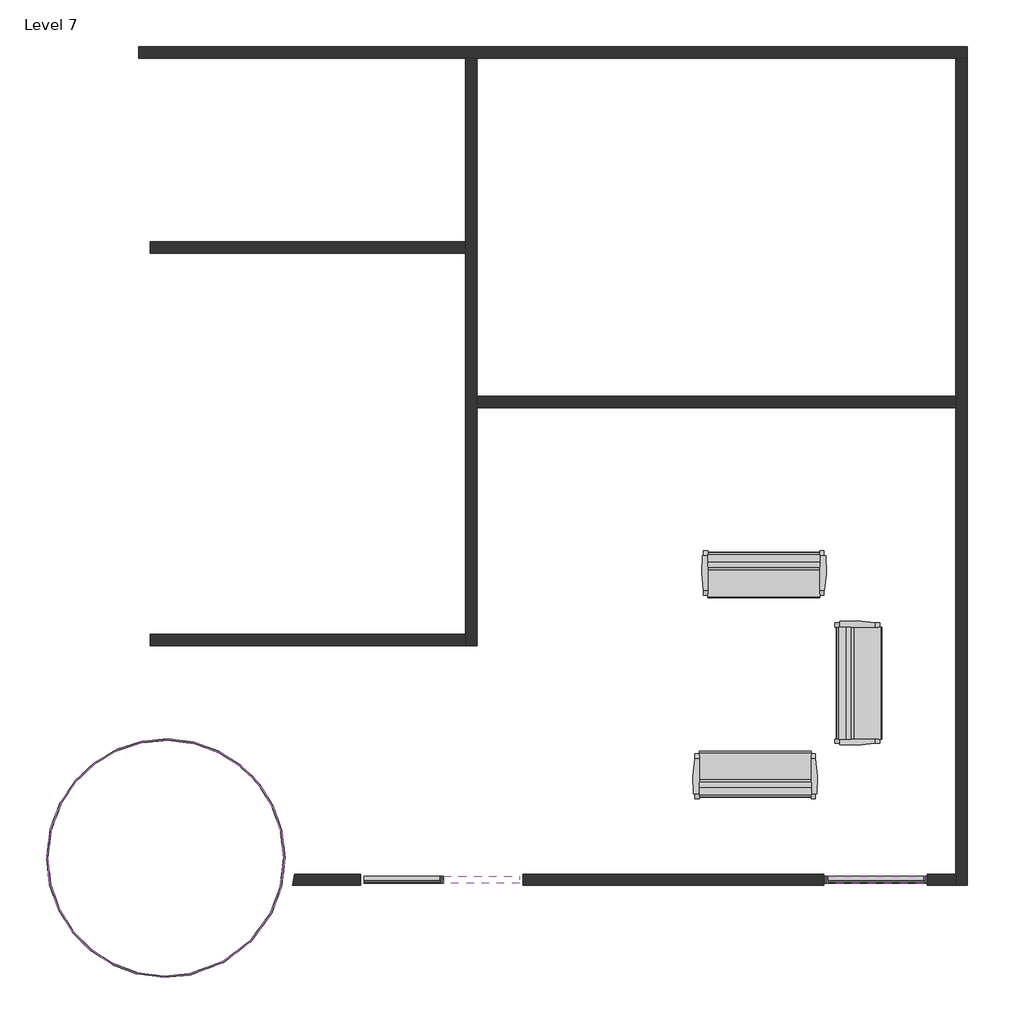
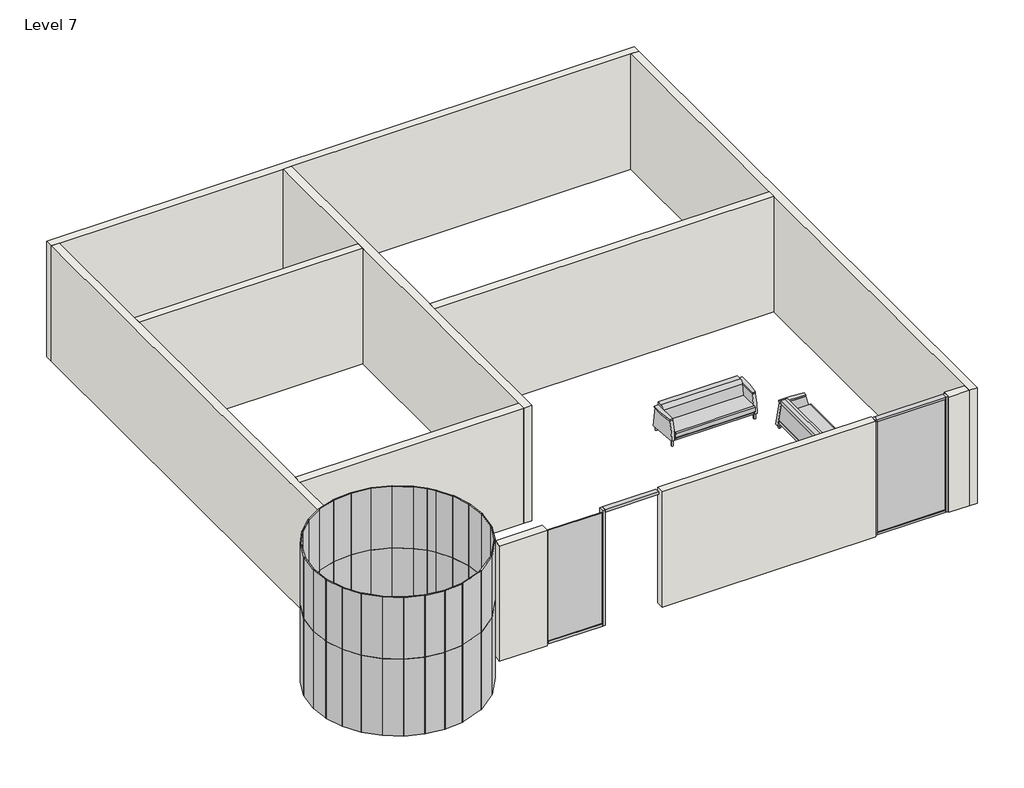
# One storey, incomplete: 58 plates, 10 walls, 7 members, 3 furniture elements.
"""IFC4 building model written with IfcOpenShell, lengths in millimetres."""

from ifc_helpers import new_model, si_unit, point, frame, frame_2d, origin, place, context, project, spatial, polyline, circle_curve, trimmed, segment, composite_curve, outline, extrude, faceted_brep, transform, mapped, element, save
from ifc_brep_helpers import plane_surface, revolved_surface, advanced_brep
from components import furniture_aff9b2fb, member_eaba9652, member_3f395ae9, member_0c868e12, member_7bc42366, system_panel_glazed_f1c144f9, system_panel_glazed_8ed2b2ee, system_panel_glazed_c7815b78, system_panel_glazed_220ba5f3, system_panel_glazed_11fb153e, system_panel_glazed_2f540b85, system_panel_glazed_4848e608, system_panel_glazed_8b35a0ff, system_panel_glazed_87282c25, system_panel_glazed_6d1bb68c, system_panel_glazed_cb3ffd69, system_panel_glazed_404d015f, system_panel_glazed_7b556abe, system_panel_glazed_370bf902

model = new_model("IFC4")

# Units and contexts
model_context = context("Model", 3, world=origin())
ifc_project = project(units=[si_unit("LENGTHUNIT", "METRE", prefix="MILLI")], contexts=[model_context])

# Site, building, storey
site = spatial("IfcSite", under=ifc_project)
building = spatial("IfcBuilding", under=site)
storey = spatial("IfcBuildingStorey", under=building, Name="Level 7", Elevation=18288.0)

# Furniture
placement = place(None, origin())
furniture_shape = furniture_aff9b2fb(model_context)
element("IfcFurniture", 1, ObjectType="Sofa-Pensi : 84\"", at=placement, inside=storey, context=model_context, shape_type="MappedRepresentation", body=[
    mapped(furniture_shape, transform((-2244.8524991, 3650.1964615, 18288.0), x_axis=(1.0, 0.0, 0.0), y_axis=(0.0, 1.0, 0.0), z_axis=(0.0, 0.0, 1.0))),
])
element("IfcFurniture", 2, ObjectType="Sofa-Pensi : 84\"", at=placement, inside=storey, context=model_context, shape_type="MappedRepresentation", body=[
    mapped(furniture_shape, transform((-12.736413, 1720.492712, 18288.0), x_axis=(0.0, 1.0, 0.0), y_axis=(-1.0, 0.0, 0.0), z_axis=(0.0, 0.0, 1.0))),
])
element("IfcFurniture", 3, ObjectType="Sofa-Pensi : 84\"", at=placement, inside=storey, context=model_context, shape_type="MappedRepresentation", body=[
    mapped(furniture_shape, transform((-1840.0399991, 648.4161336, 18288.0), x_axis=(-1.0, 0.0, 0.0), y_axis=(0.0, -1.0, 0.0), z_axis=(0.0, 0.0, 1.0))),
])

# Members
member_shape = member_eaba9652(model_context)
element("IfcMember", 4, ObjectType="Rectangular Mullion : 2.5\" x 5\" rectangular", at=placement, inside=storey, context=model_context, shape_type="MappedRepresentation", body=[
    mapped(member_shape, transform((-7672.5789001, -1482.8937024, 18288.0), x_axis=(-1.0, 0.0, 0.0), y_axis=(0.0, 1.0, 0.0), z_axis=(0.0, 0.0, -1.0))),
])
member_2_shape = member_3f395ae9(model_context)
element("IfcMember", 5, ObjectType="Rectangular Mullion : 2.5\" x 5\" rectangular", at=placement, inside=storey, context=model_context, shape_type="MappedRepresentation", body=[
    mapped(member_2_shape, transform((-899.4462491, -1482.8937024, 18288.0), x_axis=(-1.0, 0.0, 0.0), y_axis=(0.0, 1.0, 0.0), z_axis=(0.0, 0.0, -1.0))),
])
element("IfcMember", 6, ObjectType="Rectangular Mullion : 2.5\" x 5\" rectangular", at=placement, inside=storey, context=model_context, shape_type="MappedRepresentation", body=[
    mapped(member_2_shape, transform((929.3537509, -1482.8937024, 21336.0), x_axis=(1.0, 0.0, 0.0), y_axis=(0.0, 1.0, 0.0), z_axis=(0.0, 0.0, 1.0))),
])
member_3_shape = member_0c868e12(model_context)
element("IfcMember", 7, ObjectType="Rectangular Mullion : 2.5\" x 5\" rectangular", at=placement, inside=storey, context=model_context, shape_type="MappedRepresentation", body=[
    mapped(member_3_shape, transform((-7640.8289001, -1482.8937024, 21336.0), x_axis=(0.0, 0.0, 1.0), y_axis=(0.0, 1.0, 0.0), z_axis=(-1.0, 0.0, 0.0))),
])
element("IfcMember", 8, ObjectType="Rectangular Mullion : 2.5\" x 5\" rectangular", at=placement, inside=storey, context=model_context, shape_type="MappedRepresentation", body=[
    mapped(member_3_shape, transform((-7704.3289001, -1482.8937024, 18288.0), x_axis=(0.0, 0.0, -1.0), y_axis=(0.0, 1.0, 0.0), z_axis=(1.0, 0.0, 0.0))),
])
member_4_shape = member_7bc42366(model_context)
element("IfcMember", 9, ObjectType="Rectangular Mullion : 2.5\" x 5\" rectangular", at=placement, inside=storey, context=model_context, shape_type="MappedRepresentation", body=[
    mapped(member_4_shape, transform((-835.9462491, -1482.8937024, 21336.0), x_axis=(0.0, 0.0, 1.0), y_axis=(0.0, 1.0, 0.0), z_axis=(-1.0, 0.0, 0.0))),
])
element("IfcMember", 10, ObjectType="Rectangular Mullion : 2.5\" x 5\" rectangular", at=placement, inside=storey, context=model_context, shape_type="MappedRepresentation", body=[
    mapped(member_4_shape, transform((865.8537509, -1482.8937024, 18288.0), x_axis=(0.0, 0.0, -1.0), y_axis=(0.0, 1.0, 0.0), z_axis=(1.0, 0.0, 0.0))),
])

# Plates
system_panel_glazed_shape = system_panel_glazed_f1c144f9(model_context)
element("IfcPlate", 11, ObjectType="System Panel : Glazed", at=placement, inside=storey, context=model_context, shape_type="MappedRepresentation", body=[
    mapped(system_panel_glazed_shape, transform((-14541.9245022, -346.5978939, 18288.0), x_axis=(-0.3551689475306269, -0.9348021281051873, 0.0), y_axis=(0.9348021281051873, -0.3551689475306269, 0.0), z_axis=(0.0, 0.0, 1.0))),
])
element("IfcPlate", 12, ObjectType="System Panel : Glazed", at=placement, inside=storey, context=model_context, shape_type="MappedRepresentation", body=[
    mapped(system_panel_glazed_shape, transform((-10582.1178502, -1851.0877948, 18288.0), x_axis=(0.35516894753064066, 0.934802128105182, 0.0), y_axis=(-0.934802128105182, 0.35516894753064066, 0.0), z_axis=(0.0, 0.0, 1.0))),
])
element("IfcPlate", 13, ObjectType="System Panel : Glazed", at=placement, inside=storey, context=model_context, shape_type="MappedRepresentation", body=[
    mapped(system_panel_glazed_shape, transform((-10459.5232171, -1354.5613954, 18288.0), x_axis=(0.12073632210407237, 0.9926846128175765, 0.0), y_axis=(-0.9926846128175765, 0.12073632210407237, 0.0), z_axis=(0.0, 0.0, 1.0))),
])
element("IfcPlate", 14, ObjectType="System Panel : Glazed", at=placement, inside=storey, context=model_context, shape_type="MappedRepresentation", body=[
    mapped(system_panel_glazed_shape, transform((-14664.5191354, -843.1242933, 18288.0), x_axis=(-0.12073632210406239, -0.9926846128175777, 0.0), y_axis=(0.9926846128175777, -0.12073632210406239, 0.0), z_axis=(0.0, 0.0, 1.0))),
])
system_panel_glazed_2_shape = system_panel_glazed_8ed2b2ee(model_context)
element("IfcPlate", 15, ObjectType="System Panel : Glazed", at=placement, inside=storey, context=model_context, shape_type="MappedRepresentation", body=[
    mapped(system_panel_glazed_2_shape, transform((-11841.3777431, -3082.3793017, 18288.0), x_axis=(0.9398911711666007, 0.3414741371803665, 0.0), y_axis=(-0.3414741371803665, 0.9398911711666007, 0.0), z_axis=(0.0, 0.0, 1.0))),
])
element("IfcPlate", 16, ObjectType="System Panel : Glazed", at=placement, inside=storey, context=model_context, shape_type="MappedRepresentation", body=[
    mapped(system_panel_glazed_2_shape, transform((-10858.9635423, -2345.1728692, 18288.0), x_axis=(0.5905687200141164, 0.8069873524045393, 0.0), y_axis=(-0.8069873524045393, 0.5905687200141164, 0.0), z_axis=(0.0, 0.0, 1.0))),
])
element("IfcPlate", 17, ObjectType="System Panel : Glazed", at=placement, inside=storey, context=model_context, shape_type="MappedRepresentation", body=[
    mapped(system_panel_glazed_2_shape, transform((-11295.3522982, -2786.8279712, 18288.0), x_axis=(0.7998453025525061, 0.6002062078858317, 0.0), y_axis=(-0.6002062078858317, 0.7998453025525061, 0.0), z_axis=(0.0, 0.0, 1.0))),
])
system_panel_glazed_3_shape = system_panel_glazed_c7815b78(model_context)
element("IfcPlate", 18, ObjectType="System Panel : Glazed", at=placement, inside=storey, context=model_context, shape_type="MappedRepresentation", body=[
    mapped(system_panel_glazed_3_shape, transform((-10454.4737362, -864.5204039, 18288.0), x_axis=(-0.11050163420416614, 0.993875942378227, 0.0), y_axis=(-0.993875942378227, -0.11050163420416614, 0.0), z_axis=(0.0, 0.0, 1.0))),
])
element("IfcPlate", 19, ObjectType="System Panel : Glazed", at=placement, inside=storey, context=model_context, shape_type="MappedRepresentation", body=[
    mapped(system_panel_glazed_3_shape, transform((-14669.5686163, -1333.1652848, 18288.0), x_axis=(0.11050163420415136, -0.9938759423782286, 0.0), y_axis=(0.9938759423782286, 0.11050163420415136, 0.0), z_axis=(0.0, 0.0, 1.0))),
])
element("IfcPlate", 20, ObjectType="System Panel : Glazed", at=placement, inside=storey, context=model_context, shape_type="MappedRepresentation", body=[
    mapped(system_panel_glazed_3_shape, transform((-11410.1424167, 681.5611944, 18288.0), x_axis=(-0.8396018558176894, 0.5432022861766066, 0.0), y_axis=(-0.5432022861766066, -0.8396018558176894, 0.0), z_axis=(0.0, 0.0, 1.0))),
])
element("IfcPlate", 21, ObjectType="System Panel : Glazed", at=placement, inside=storey, context=model_context, shape_type="MappedRepresentation", body=[
    mapped(system_panel_glazed_3_shape, transform((-13212.0893695, 919.590846, 18288.0), x_axis=(-0.9518517343814786, -0.3065587639506839, 0.0), y_axis=(0.3065587639506839, -0.9518517343814786, 0.0), z_axis=(0.0, 0.0, 1.0))),
])
element("IfcPlate", 22, ObjectType="System Panel : Glazed", at=placement, inside=storey, context=model_context, shape_type="MappedRepresentation", body=[
    mapped(system_panel_glazed_3_shape, transform((-12839.7224363, -3201.1142893, 18288.0), x_axis=(0.9913878918151698, -0.1309581916577702, 0.0), y_axis=(0.1309581916577702, 0.9913878918151698, 0.0), z_axis=(0.0, 0.0, 1.0))),
])
element("IfcPlate", 23, ObjectType="System Panel : Glazed", at=placement, inside=storey, context=model_context, shape_type="MappedRepresentation", body=[
    mapped(system_panel_glazed_3_shape, transform((-14365.783041, -2213.7896382, 18288.0), x_axis=(0.5257859322352114, -0.8506169252157811, 0.0), y_axis=(0.8506169252157811, 0.5257859322352114, 0.0), z_axis=(0.0, 0.0, 1.0))),
])
element("IfcPlate", 24, ObjectType="System Panel : Glazed", at=placement, inside=storey, context=model_context, shape_type="MappedRepresentation", body=[
    mapped(system_panel_glazed_3_shape, transform((-13713.8999358, -2879.2468831, 18288.0), x_axis=(0.8396018558176805, -0.5432022861766201, 0.0), y_axis=(0.5432022861766201, 0.8396018558176805, 0.0), z_axis=(0.0, 0.0, 1.0))),
])
element("IfcPlate", 25, ObjectType="System Panel : Glazed", at=placement, inside=storey, context=model_context, shape_type="MappedRepresentation", body=[
    mapped(system_panel_glazed_3_shape, transform((-14014.4059364, 446.2272921, 18288.0), x_axis=(-0.7286232370002992, -0.6849147235263715, 0.0), y_axis=(0.6849147235263715, -0.7286232370002992, 0.0), z_axis=(0.0, 0.0, 1.0))),
])
element("IfcPlate", 26, ObjectType="System Panel : Glazed", at=placement, inside=storey, context=model_context, shape_type="MappedRepresentation", body=[
    mapped(system_panel_glazed_3_shape, transform((-12284.3199161, 1003.4286006, 18288.0), x_axis=(-0.9913878918151723, 0.13095819165775144, 0.0), y_axis=(-0.13095819165775144, -0.9913878918151723, 0.0), z_axis=(0.0, 0.0, 1.0))),
])
element("IfcPlate", 27, ObjectType="System Panel : Glazed", at=placement, inside=storey, context=model_context, shape_type="MappedRepresentation", body=[
    mapped(system_panel_glazed_3_shape, transform((-12752.8652893, 1013.0855973, 18288.0), x_axis=(-0.9959419324521102, -0.08999815100076568, 0.0), y_axis=(0.08999815100076568, -0.9959419324521102, 0.0), z_axis=(0.0, 0.0, 1.0))),
])
element("IfcPlate", 28, ObjectType="System Panel : Glazed", at=placement, inside=storey, context=model_context, shape_type="MappedRepresentation", body=[
    mapped(system_panel_glazed_3_shape, transform((-11829.3381514, 891.0915272, 18288.0), x_axis=(-0.9384120429483949, 0.3455182160891376, 0.0), y_axis=(-0.3455182160891376, -0.9384120429483949, 0.0), z_axis=(0.0, 0.0, 1.0))),
])
element("IfcPlate", 29, ObjectType="System Panel : Glazed", at=placement, inside=storey, context=model_context, shape_type="MappedRepresentation", body=[
    mapped(system_panel_glazed_3_shape, transform((-10557.4115054, -407.3204039, 18288.0), x_axis=(-0.3261077326604367, 0.9453326116764772, 0.0), y_axis=(-0.9453326116764772, -0.3261077326604367, 0.0), z_axis=(0.0, 0.0, 1.0))),
])
element("IfcPlate", 30, ObjectType="System Panel : Glazed", at=placement, inside=storey, context=model_context, shape_type="MappedRepresentation", body=[
    mapped(system_panel_glazed_3_shape, transform((-12371.1770631, -3210.771286, 18288.0), x_axis=(0.9959419324521115, 0.08999815100075001, 0.0), y_axis=(-0.08999815100075001, 0.9959419324521115, 0.0), z_axis=(0.0, 0.0, 1.0))),
])
element("IfcPlate", 31, ObjectType="System Panel : Glazed", at=placement, inside=storey, context=model_context, shape_type="MappedRepresentation", body=[
    mapped(system_panel_glazed_3_shape, transform((-13294.7042011, -3088.7772159, 18288.0), x_axis=(0.9384120429483891, -0.34551821608915334, 0.0), y_axis=(0.34551821608915334, 0.9384120429483891, 0.0), z_axis=(0.0, 0.0, 1.0))),
])
element("IfcPlate", 32, ObjectType="System Panel : Glazed", at=placement, inside=storey, context=model_context, shape_type="MappedRepresentation", body=[
    mapped(system_panel_glazed_3_shape, transform((-14076.8350959, -2582.7572647, 18288.0), x_axis=(0.6997834615185511, -0.7143550286692988, 0.0), y_axis=(0.7143550286692988, 0.6997834615185511, 0.0), z_axis=(0.0, 0.0, 1.0))),
])
element("IfcPlate", 33, ObjectType="System Panel : Glazed", at=placement, inside=storey, context=model_context, shape_type="MappedRepresentation", body=[
    mapped(system_panel_glazed_3_shape, transform((-14566.6308471, -1790.3652848, 18288.0), x_axis=(0.32610773266042153, -0.9453326116764824, 0.0), y_axis=(0.9453326116764824, 0.32610773266042153, 0.0), z_axis=(0.0, 0.0, 1.0))),
])
element("IfcPlate", 34, ObjectType="System Panel : Glazed", at=placement, inside=storey, context=model_context, shape_type="MappedRepresentation", body=[
    mapped(system_panel_glazed_3_shape, transform((-14318.3113206, 89.4787227, 18288.0), x_axis=(-0.5603879632167612, -0.8282302401396425, 0.0), y_axis=(0.8282302401396425, -0.5603879632167612, 0.0), z_axis=(0.0, 0.0, 1.0))),
])
element("IfcPlate", 35, ObjectType="System Panel : Glazed", at=placement, inside=storey, context=model_context, shape_type="MappedRepresentation", body=[
    mapped(system_panel_glazed_3_shape, transform((-13639.5625299, 727.5108588, 18288.0), x_axis=(-0.8612707706620224, -0.5081462974412448, 0.0), y_axis=(0.5081462974412448, -0.8612707706620224, 0.0), z_axis=(0.0, 0.0, 1.0))),
])
system_panel_glazed_4_shape = system_panel_glazed_220ba5f3(model_context)
element("IfcPlate", 36, ObjectType="System Panel : Glazed", at=placement, inside=storey, context=model_context, shape_type="MappedRepresentation", body=[
    mapped(system_panel_glazed_4_shape, transform((-10742.3305673, -4.7597883, 18288.0), x_axis=(-0.5152811917631037, 0.8570211744263939, 0.0), y_axis=(-0.8570211744263939, -0.5152811917631037, 0.0), z_axis=(0.0, 0.0, 1.0))),
])
system_panel_glazed_5_shape = system_panel_glazed_11fb153e(model_context)
element("IfcPlate", 37, ObjectType="System Panel : Glazed", at=placement, inside=storey, context=model_context, shape_type="MappedRepresentation", body=[
    mapped(system_panel_glazed_5_shape, transform((-11098.0043985, 445.2241463, 18288.0), x_axis=(-0.7256671855033587, 0.6880458821064435, 0.0), y_axis=(-0.6880458821064435, -0.7256671855033587, 0.0), z_axis=(0.0, 0.0, 1.0))),
])
system_panel_glazed_6_shape = system_panel_glazed_2f540b85(model_context)
element("IfcPlate", 38, ObjectType="System Panel : Glazed", at=placement, inside=storey, context=model_context, shape_type="MappedRepresentation", body=[
    mapped(system_panel_glazed_6_shape, transform((-10917.0903061, 255.9395759, 18288.0), x_axis=(-0.6357445726375757, 0.7718995001694627, 0.0), y_axis=(-0.7718995001694627, -0.6357445726375757, 0.0), z_axis=(0.0, 0.0, 1.0))),
])
system_panel_glazed_7_shape = system_panel_glazed_4848e608(model_context)
element("IfcPlate", 39, ObjectType="System Panel : Glazed", at=placement, inside=storey, context=model_context, shape_type="MappedRepresentation", body=[
    mapped(system_panel_glazed_7_shape, transform((-14669.5686163, -1333.1652848, 20320.0), x_axis=(0.11050163420415136, -0.9938759423782286, 0.0), y_axis=(0.9938759423782286, 0.11050163420415136, 0.0), z_axis=(0.0, 0.0, 1.0))),
])
element("IfcPlate", 40, ObjectType="System Panel : Glazed", at=placement, inside=storey, context=model_context, shape_type="MappedRepresentation", body=[
    mapped(system_panel_glazed_7_shape, transform((-14365.783041, -2213.7896382, 20320.0), x_axis=(0.5257859322352114, -0.8506169252157811, 0.0), y_axis=(0.8506169252157811, 0.5257859322352114, 0.0), z_axis=(0.0, 0.0, 1.0))),
])
element("IfcPlate", 41, ObjectType="System Panel : Glazed", at=placement, inside=storey, context=model_context, shape_type="MappedRepresentation", body=[
    mapped(system_panel_glazed_7_shape, transform((-13713.8999358, -2879.2468831, 20320.0), x_axis=(0.8396018558176805, -0.5432022861766201, 0.0), y_axis=(0.5432022861766201, 0.8396018558176805, 0.0), z_axis=(0.0, 0.0, 1.0))),
])
element("IfcPlate", 42, ObjectType="System Panel : Glazed", at=placement, inside=storey, context=model_context, shape_type="MappedRepresentation", body=[
    mapped(system_panel_glazed_7_shape, transform((-12839.7224363, -3201.1142893, 20320.0), x_axis=(0.9913878918151698, -0.13095819165777017, 0.0), y_axis=(0.13095819165777017, 0.9913878918151698, 0.0), z_axis=(0.0, 0.0, 1.0))),
])
element("IfcPlate", 43, ObjectType="System Panel : Glazed", at=placement, inside=storey, context=model_context, shape_type="MappedRepresentation", body=[
    mapped(system_panel_glazed_7_shape, transform((-12371.1770631, -3210.771286, 20320.0), x_axis=(0.9959419324521115, 0.08999815100075001, 0.0), y_axis=(-0.08999815100075001, 0.9959419324521115, 0.0), z_axis=(0.0, 0.0, 1.0))),
])
element("IfcPlate", 44, ObjectType="System Panel : Glazed", at=placement, inside=storey, context=model_context, shape_type="MappedRepresentation", body=[
    mapped(system_panel_glazed_7_shape, transform((-13294.7042011, -3088.7772159, 20320.0), x_axis=(0.9384120429483891, -0.34551821608915334, 0.0), y_axis=(0.34551821608915334, 0.9384120429483891, 0.0), z_axis=(0.0, 0.0, 1.0))),
])
element("IfcPlate", 45, ObjectType="System Panel : Glazed", at=placement, inside=storey, context=model_context, shape_type="MappedRepresentation", body=[
    mapped(system_panel_glazed_7_shape, transform((-14076.8350959, -2582.7572647, 20320.0), x_axis=(0.6997834615185511, -0.7143550286692988, 0.0), y_axis=(0.7143550286692988, 0.6997834615185511, 0.0), z_axis=(0.0, 0.0, 1.0))),
])
element("IfcPlate", 46, ObjectType="System Panel : Glazed", at=placement, inside=storey, context=model_context, shape_type="MappedRepresentation", body=[
    mapped(system_panel_glazed_7_shape, transform((-14566.6308471, -1790.3652848, 20320.0), x_axis=(0.32610773266042153, -0.9453326116764824, 0.0), y_axis=(0.9453326116764824, 0.32610773266042153, 0.0), z_axis=(0.0, 0.0, 1.0))),
])
element("IfcPlate", 47, ObjectType="System Panel : Glazed", at=placement, inside=storey, context=model_context, shape_type="MappedRepresentation", body=[
    mapped(system_panel_glazed_7_shape, transform((-10454.4737362, -864.5204039, 20320.0), x_axis=(-0.11050163420416614, 0.993875942378227, 0.0), y_axis=(-0.993875942378227, -0.11050163420416614, 0.0), z_axis=(0.0, 0.0, 1.0))),
])
element("IfcPlate", 48, ObjectType="System Panel : Glazed", at=placement, inside=storey, context=model_context, shape_type="MappedRepresentation", body=[
    mapped(system_panel_glazed_7_shape, transform((-10557.4115054, -407.3204039, 20320.0), x_axis=(-0.3261077326604368, 0.9453326116764772, 0.0), y_axis=(-0.9453326116764772, -0.3261077326604368, 0.0), z_axis=(0.0, 0.0, 1.0))),
])
element("IfcPlate", 49, ObjectType="System Panel : Glazed", at=placement, inside=storey, context=model_context, shape_type="MappedRepresentation", body=[
    mapped(system_panel_glazed_7_shape, transform((-11410.1424167, 681.5611944, 20320.0), x_axis=(-0.8396018558176894, 0.5432022861766066, 0.0), y_axis=(-0.5432022861766066, -0.8396018558176894, 0.0), z_axis=(0.0, 0.0, 1.0))),
])
element("IfcPlate", 50, ObjectType="System Panel : Glazed", at=placement, inside=storey, context=model_context, shape_type="MappedRepresentation", body=[
    mapped(system_panel_glazed_7_shape, transform((-11829.3381514, 891.0915272, 20320.0), x_axis=(-0.9384120429483949, 0.3455182160891376, 0.0), y_axis=(-0.3455182160891376, -0.9384120429483949, 0.0), z_axis=(0.0, 0.0, 1.0))),
])
element("IfcPlate", 51, ObjectType="System Panel : Glazed", at=placement, inside=storey, context=model_context, shape_type="MappedRepresentation", body=[
    mapped(system_panel_glazed_7_shape, transform((-12284.3199161, 1003.4286006, 20320.0), x_axis=(-0.9913878918151723, 0.1309581916577514, 0.0), y_axis=(-0.1309581916577514, -0.9913878918151723, 0.0), z_axis=(0.0, 0.0, 1.0))),
])
element("IfcPlate", 52, ObjectType="System Panel : Glazed", at=placement, inside=storey, context=model_context, shape_type="MappedRepresentation", body=[
    mapped(system_panel_glazed_7_shape, transform((-12752.8652893, 1013.0855973, 20320.0), x_axis=(-0.9959419324521102, -0.08999815100076568, 0.0), y_axis=(0.08999815100076568, -0.9959419324521102, 0.0), z_axis=(0.0, 0.0, 1.0))),
])
element("IfcPlate", 53, ObjectType="System Panel : Glazed", at=placement, inside=storey, context=model_context, shape_type="MappedRepresentation", body=[
    mapped(system_panel_glazed_7_shape, transform((-13212.0893695, 919.590846, 20320.0), x_axis=(-0.9518517343814786, -0.3065587639506839, 0.0), y_axis=(0.3065587639506839, -0.9518517343814786, 0.0), z_axis=(0.0, 0.0, 1.0))),
])
element("IfcPlate", 54, ObjectType="System Panel : Glazed", at=placement, inside=storey, context=model_context, shape_type="MappedRepresentation", body=[
    mapped(system_panel_glazed_7_shape, transform((-13639.5625299, 727.5108588, 20320.0), x_axis=(-0.8612707706620223, -0.508146297441245, 0.0), y_axis=(0.508146297441245, -0.8612707706620223, 0.0), z_axis=(0.0, 0.0, 1.0))),
])
element("IfcPlate", 55, ObjectType="System Panel : Glazed", at=placement, inside=storey, context=model_context, shape_type="MappedRepresentation", body=[
    mapped(system_panel_glazed_7_shape, transform((-14014.4059364, 446.2272921, 20320.0), x_axis=(-0.7286232370002992, -0.6849147235263715, 0.0), y_axis=(0.6849147235263715, -0.7286232370002992, 0.0), z_axis=(0.0, 0.0, 1.0))),
])
element("IfcPlate", 56, ObjectType="System Panel : Glazed", at=placement, inside=storey, context=model_context, shape_type="MappedRepresentation", body=[
    mapped(system_panel_glazed_7_shape, transform((-14318.3113206, 89.4787227, 20320.0), x_axis=(-0.5603879632167612, -0.8282302401396425, 0.0), y_axis=(0.8282302401396425, -0.5603879632167612, 0.0), z_axis=(0.0, 0.0, 1.0))),
])
system_panel_glazed_8_shape = system_panel_glazed_8b35a0ff(model_context)
element("IfcPlate", 57, ObjectType="System Panel : Glazed", at=placement, inside=storey, context=model_context, shape_type="MappedRepresentation", body=[
    mapped(system_panel_glazed_8_shape, transform((-10742.3305673, -4.7597883, 20320.0), x_axis=(-0.5152811917631037, 0.8570211744263939, 0.0), y_axis=(-0.8570211744263939, -0.5152811917631037, 0.0), z_axis=(0.0, 0.0, 1.0))),
])
system_panel_glazed_9_shape = system_panel_glazed_87282c25(model_context)
element("IfcPlate", 58, ObjectType="System Panel : Glazed", at=placement, inside=storey, context=model_context, shape_type="MappedRepresentation", body=[
    mapped(system_panel_glazed_9_shape, transform((-10917.0903061, 255.9395759, 20320.0), x_axis=(-0.6357445726375757, 0.7718995001694627, 0.0), y_axis=(-0.7718995001694627, -0.6357445726375757, 0.0), z_axis=(0.0, 0.0, 1.0))),
])
system_panel_glazed_10_shape = system_panel_glazed_6d1bb68c(model_context)
element("IfcPlate", 59, ObjectType="System Panel : Glazed", at=placement, inside=storey, context=model_context, shape_type="MappedRepresentation", body=[
    mapped(system_panel_glazed_10_shape, transform((-11098.0043985, 445.2241463, 20320.0), x_axis=(-0.7256671855033587, 0.6880458821064435, 0.0), y_axis=(-0.6880458821064435, -0.7256671855033587, 0.0), z_axis=(0.0, 0.0, 1.0))),
])
system_panel_glazed_11_shape = system_panel_glazed_cb3ffd69(model_context)
element("IfcPlate", 60, ObjectType="System Panel : Glazed", at=placement, inside=storey, context=model_context, shape_type="MappedRepresentation", body=[
    mapped(system_panel_glazed_11_shape, transform((-10582.1178502, -1851.0877948, 20320.0), x_axis=(0.35516894753064066, 0.934802128105182, 0.0), y_axis=(-0.934802128105182, 0.35516894753064066, 0.0), z_axis=(0.0, 0.0, 1.0))),
])
element("IfcPlate", 61, ObjectType="System Panel : Glazed", at=placement, inside=storey, context=model_context, shape_type="MappedRepresentation", body=[
    mapped(system_panel_glazed_11_shape, transform((-10459.5232171, -1354.5613954, 20320.0), x_axis=(0.1207363221040724, 0.9926846128175765, 0.0), y_axis=(-0.9926846128175765, 0.1207363221040724, 0.0), z_axis=(0.0, 0.0, 1.0))),
])
element("IfcPlate", 62, ObjectType="System Panel : Glazed", at=placement, inside=storey, context=model_context, shape_type="MappedRepresentation", body=[
    mapped(system_panel_glazed_11_shape, transform((-14541.9245022, -346.5978939, 20320.0), x_axis=(-0.3551689475306269, -0.9348021281051873, 0.0), y_axis=(0.9348021281051873, -0.3551689475306269, 0.0), z_axis=(0.0, 0.0, 1.0))),
])
element("IfcPlate", 63, ObjectType="System Panel : Glazed", at=placement, inside=storey, context=model_context, shape_type="MappedRepresentation", body=[
    mapped(system_panel_glazed_11_shape, transform((-14664.5191354, -843.1242933, 20320.0), x_axis=(-0.1207363221040624, -0.9926846128175777, 0.0), y_axis=(0.9926846128175777, -0.1207363221040624, 0.0), z_axis=(0.0, 0.0, 1.0))),
])
system_panel_glazed_12_shape = system_panel_glazed_404d015f(model_context)
element("IfcPlate", 64, ObjectType="System Panel : Glazed", at=placement, inside=storey, context=model_context, shape_type="MappedRepresentation", body=[
    mapped(system_panel_glazed_12_shape, transform((-11841.3777431, -3082.3793017, 20320.0), x_axis=(0.9398911711666007, 0.3414741371803665, 0.0), y_axis=(-0.3414741371803665, 0.9398911711666007, 0.0), z_axis=(0.0, 0.0, 1.0))),
])
element("IfcPlate", 65, ObjectType="System Panel : Glazed", at=placement, inside=storey, context=model_context, shape_type="MappedRepresentation", body=[
    mapped(system_panel_glazed_12_shape, transform((-10858.9635423, -2345.1728692, 20320.0), x_axis=(0.5905687200141164, 0.8069873524045393, 0.0), y_axis=(-0.8069873524045393, 0.5905687200141164, 0.0), z_axis=(0.0, 0.0, 1.0))),
])
element("IfcPlate", 66, ObjectType="System Panel : Glazed", at=placement, inside=storey, context=model_context, shape_type="MappedRepresentation", body=[
    mapped(system_panel_glazed_12_shape, transform((-11295.3522982, -2786.8279712, 20320.0), x_axis=(0.7998453025525062, 0.6002062078858316, 0.0), y_axis=(-0.6002062078858316, 0.7998453025525062, 0.0), z_axis=(0.0, 0.0, 1.0))),
])
system_panel_glazed_13_shape = system_panel_glazed_7b556abe(model_context)
element("IfcPlate", 67, ObjectType="System Panel : Glazed", at=placement, inside=storey, context=model_context, shape_type="MappedRepresentation", body=[
    mapped(system_panel_glazed_13_shape, transform((-8376.2702257, -1482.8937024, 18351.5), x_axis=(-1.0, 0.0, 0.0), y_axis=(0.0, -1.0, 0.0), z_axis=(0.0, 0.0, 1.0))),
])
system_panel_glazed_14_shape = system_panel_glazed_370bf902(model_context)
element("IfcPlate", 68, ObjectType="System Panel : Glazed", at=placement, inside=storey, context=model_context, shape_type="MappedRepresentation", body=[
    mapped(system_panel_glazed_14_shape, transform((14.9537509, -1482.8937024, 18351.5), x_axis=(-1.0, 0.0, 0.0), y_axis=(0.0, -1.0, 0.0), z_axis=(0.0, 0.0, 1.0))),
])

# Walls
element("IfcWall", 69, ObjectType="Generic - 8\"", at=placement, inside=storey, context=model_context, shape_type="Brep", body=[
    faceted_brep([(-13040.6462491, 13071.3062976, 18288.0), (-12837.4462491, 13071.3062976, 18288.0), (-7249.4462491, 13071.3062976, 18288.0), (-7046.2462491, 13071.3062976, 18288.0), (1437.3537509, 13071.3062976, 18288.0), (1640.5537509, 13071.3062976, 18288.0), (1640.5537509, 13071.3062976, 21336.0), (1437.3537509, 13071.3062976, 21336.0), (-7046.2462491, 13071.3062976, 21336.0), (-7249.4462491, 13071.3062976, 21336.0), (-12837.4462491, 13071.3062976, 21336.0), (-13040.6462491, 13071.3062976, 21336.0), (-13040.6462491, 13274.5062976, 18288.0), (-13040.6462491, 13274.5062976, 21336.0), (1640.5537509, 13274.5062976, 21336.0), (1640.5537509, 13274.5062976, 18288.0)], [[[0, 1, 2, 3, 4, 5, 6, 7, 8, 9, 10, 11]], [[12, 13, 14, 15]], [[5, 4, 3, 2, 1, 0, 12, 15]], [[11, 10, 9, 8, 7, 6, 14, 13]], [[6, 5, 15, 14]], [[0, 11, 13, 12]]]),
])
element("IfcWall", 70, ObjectType="Generic - 8\"", at=placement, inside=storey, context=model_context, shape_type="Brep", body=[
    faceted_brep([(1437.3537509, 13071.3062976, 18288.0), (1437.3537509, 7076.9062976, 18288.0), (1437.3537509, 6873.7062976, 18288.0), (1437.3537509, -1381.2937024, 18288.0), (1437.3537509, -1584.4937024, 18288.0), (1437.3537509, -1584.4937024, 21336.0), (1437.3537509, -1381.2937024, 21336.0), (1437.3537509, 6873.7062976, 21336.0), (1437.3537509, 7076.9062976, 21336.0), (1437.3537509, 13071.3062976, 21336.0), (1640.5537509, 13071.3062976, 18288.0), (1640.5537509, 13071.3062976, 21336.0), (1640.5537509, -1584.4937024, 21336.0), (1640.5537509, -1584.4937024, 18288.0)], [[[0, 1, 2, 3, 4, 5, 6, 7, 8, 9]], [[10, 11, 12, 13]], [[4, 3, 2, 1, 0, 10, 13]], [[9, 8, 7, 6, 5, 12, 11]], [[0, 9, 11, 10]], [[5, 4, 13, 12]]]),
])
element("IfcWall", 71, ObjectType="Generic - 8\"", at=placement, inside=storey, context=model_context, shape_type="AdvancedBrep", body=[
    advanced_brep(
    [(-13040.6462491, 13071.3062976, 18288.0), (-13040.6462491, 1241.1937063, 18288.0), (-13040.6462491, 1241.1937063, 21336.0), (-13040.6462491, 13071.3062976, 21336.0), (-12837.4462491, 13071.3062976, 18288.0), (-12837.4462491, 13071.3062976, 21336.0), (-12837.4462491, 9820.1062976, 21336.0), (-12837.4462491, 9616.9062976, 21336.0), (-12837.4462491, 2862.698962, 21336.0), (-12837.4462491, 2659.498962, 21336.0), (-12837.4462491, 1269.6553935, 21336.0), (-12837.4462491, 1269.6553935, 18288.0), (-12837.4462491, 2659.498962, 18288.0), (-12837.4462491, 2862.698962, 18288.0), (-12837.4462491, 9616.9062976, 18288.0), (-12837.4462491, 9820.1062976, 18288.0)],
    [
        (0, 1),
        (1, 2),
        (2, 3),
        (3, 0),
        (4, 5),
        (5, 6),
        (6, 7),
        (7, 8),
        (8, 9),
        (9, 10),
        (10, 11),
        (11, 12),
        (12, 13),
        (13, 14),
        (14, 15),
        (15, 4),
        (0, 4),
        (11, 1, circle_curve(frame((-12612.6150686, -1075.1054509, 18288.0), z_axis=(0.0, 0.0, 1.0), x_axis=(1.0, 0.0, 0.0)), 2355.5153315)),
        (2, 10, circle_curve(frame((-12612.6150686, -1075.1054509, 21336.0), z_axis=(0.0, 0.0, -1.0), x_axis=(1.0, 0.0, 0.0)), 2355.5153315)),
        (5, 3),
    ],
    [
        plane_surface(frame((-13040.6462491, 16068.5062976, 18288.0), z_axis=(-1.0, 0.0, 0.0), x_axis=(0.0, -1.0, 0.0))),
        plane_surface(frame((-12837.4462491, 16068.5062976, 18288.0), z_axis=(1.0, 0.0, 0.0), x_axis=(0.0, 1.0, 0.0))),
        plane_surface(frame((-13040.6462491, 13172.9062976, 18288.0), z_axis=(0.0, 0.0, -1.0), x_axis=(1.0, 0.0, 0.0))),
        plane_surface(frame((-13040.6462491, 1155.046339, 21336.0), z_axis=(0.0, 0.0, 1.0), x_axis=(1.0, 0.0, 0.0))),
        plane_surface(frame((-16139.4462491, 13071.3062976, 18288.0), z_axis=(0.0, 1.0, 0.0), x_axis=(1.0, 0.0, 0.0))),
        revolved_surface(polyline([(-10257.099737100001, -1075.1054509, 21336.0), (-10257.099737100001, -1075.1054509, 18288.0)]), (-12612.6150686, -1075.1054509, 18288.0), (0.0, 0.0, 1.0)),
    ],
    [
        (0, [[1, 2, 3, 4]]),
        (1, [[5, 6, 7, 8, 9, 10, 11, 12, 13, 14, 15, 16]]),
        (2, [[-1, 17, -16, -15, -14, -13, -12, 18]]),
        (3, [[-3, 19, -10, -9, -8, -7, -6, 20]]),
        (4, [[-4, -20, -5, -17]]),
        (5, [[-2, -18, -11, -19]]),
    ],
),
])
element("IfcWall", 72, ObjectType="Generic - 8\"", at=placement, inside=storey, context=model_context, shape_type="Brep", body=[
    faceted_brep([(-7249.4462491, 13071.3062976, 18288.0), (-7249.4462491, 9820.1062976, 18288.0), (-7249.4462491, 9616.9062976, 18288.0), (-7249.4462491, 2862.698962, 18288.0), (-7249.4462491, 2659.498962, 18288.0), (-7249.4462491, 2659.498962, 21336.0), (-7249.4462491, 2862.698962, 21336.0), (-7249.4462491, 9616.9062976, 21336.0), (-7249.4462491, 9820.1062976, 21336.0), (-7249.4462491, 13071.3062976, 21336.0), (-7046.2462491, 13071.3062976, 18288.0), (-7046.2462491, 13071.3062976, 21336.0), (-7046.2462491, 7076.9062976, 21336.0), (-7046.2462491, 6873.7062976, 21336.0), (-7046.2462491, 2659.498962, 21336.0), (-7046.2462491, 2659.498962, 18288.0), (-7046.2462491, 6873.7062976, 18288.0), (-7046.2462491, 7076.9062976, 18288.0)], [[[0, 1, 2, 3, 4, 5, 6, 7, 8, 9]], [[10, 11, 12, 13, 14, 15, 16, 17]], [[4, 3, 2, 1, 0, 10, 17, 16, 15]], [[9, 8, 7, 6, 5, 14, 13, 12, 11]], [[0, 9, 11, 10]], [[5, 4, 15, 14]]]),
])
element("IfcWall", 73, ObjectType="Generic - 8\"", at=placement, inside=storey, context=model_context, shape_type="SweptSolid", body=[
    extrude(outline(polyline([(1437.3537509, 6873.7062976), (-7046.2462491, 6873.7062976), (-7046.2462491, 7076.9062976), (1437.3537509, 7076.9062976), (1437.3537509, 6873.7062976)])), frame((0.0, 0.0, 18288.0), z_axis=(0.0, 0.0, 1.0), x_axis=(1.0, 0.0, 0.0)), (0.0, 0.0, 1.0), 3048.0),
])
element("IfcWall", 74, ObjectType="Generic - 8\"", at=placement, inside=storey, context=model_context, shape_type="SweptSolid", body=[
    extrude(outline(polyline([(-12837.4462491, 9820.1062976), (-7249.4462491, 9820.1062976), (-7249.4462491, 9616.9062976), (-12837.4462491, 9616.9062976), (-12837.4462491, 9820.1062976)])), frame((0.0, 0.0, 18288.0), z_axis=(0.0, 0.0, 1.0), x_axis=(1.0, 0.0, 0.0)), (0.0, 0.0, 1.0), 3048.0),
])
element("IfcWall", 75, ObjectType="Generic - 8\"", at=placement, inside=storey, context=model_context, shape_type="SweptSolid", body=[
    extrude(outline(polyline([(-12837.4462491, 2862.698962), (-7249.4462491, 2862.698962), (-7249.4462491, 2659.498962), (-12837.4462491, 2659.498962), (-12837.4462491, 2862.698962)])), frame((0.0, 0.0, 18288.0), z_axis=(0.0, 0.0, 1.0), x_axis=(1.0, 0.0, 0.0)), (0.0, 0.0, 1.0), 3048.0),
])
element("IfcWall", 76, ObjectType="Generic - 8\"", at=placement, inside=storey, context=model_context, shape_type="SweptSolid", body=[
    extrude(outline(composite_curve([segment(polyline([(-9111.7115512, -1584.4937024), (-10312.8376694, -1584.4937024)]), True, "CONTINUOUS"), segment(trimmed(circle_curve(frame_2d((-12612.6150686, -1075.1054509)), 2355.5153315), [point((-10312.8376694, -1584.4937024))], [point((-10277.0848865, -1381.2937024))], True, "CARTESIAN"), True, "CONTINUOUS"), segment(polyline([(-10277.0848865, -1381.2937024), (-9111.7115512, -1381.2937024), (-9111.7115512, -1584.4937024)]), True, "CONTINUOUS")], self_intersect=False)), frame((0.0, 0.0, 18288.0), z_axis=(0.0, 0.0, 1.0), x_axis=(1.0, 0.0, 0.0)), (0.0, 0.0, 1.0), 3048.0),
])
element("IfcWall", 77, ObjectType="Generic - 8\"", at=placement, inside=storey, context=model_context, shape_type="SweptSolid", body=[
    extrude(outline(polyline([(-899.4462491, -1584.4937024), (-6233.4462491, -1584.4937024), (-6233.4462491, -1381.2937024), (-899.4462491, -1381.2937024), (-899.4462491, -1584.4937024)])), frame((0.0, 0.0, 18288.0), z_axis=(0.0, 0.0, 1.0), x_axis=(1.0, 0.0, 0.0)), (0.0, 0.0, 1.0), 3048.0),
])
element("IfcWall", 78, ObjectType="Generic - 8\"", at=placement, inside=storey, context=model_context, shape_type="SweptSolid", body=[
    extrude(outline(polyline([(929.3537509, -1381.2937024), (1437.3537509, -1381.2937024), (1437.3537509, -1584.4937024), (929.3537509, -1584.4937024), (929.3537509, -1381.2937024)])), frame((0.0, 0.0, 18288.0), z_axis=(0.0, 0.0, 1.0), x_axis=(1.0, 0.0, 0.0)), (0.0, 0.0, 1.0), 3048.0),
])

save(model, "model.ifc")

# Revit data of these elements
# Type "Sofa-Pensi : 84\""
#   Assembly Code = "E2020200"
#   Length = 7' - 0"
#   Frame Material = Cherry
#   Seat Material = Linen, Beige
#   Feet Material = Steel, Chrome Plated
#   Default Elevation = 0
# Type "Rectangular Mullion : 2.5\" x 5\" rectangular"
#   built-in parameter 1007304 = 0.416667 (stored number, unit not read)
#   built-in parameter 1007301 = 0.104167 (stored number, unit not read)
#   built-in parameter 1007300 = 0.104167 (stored number, unit not read)
# Type "System Panel : Glazed"
#   Construction Type Id = "GSP4R"
#   Analytic Construction = "1/8 in Pilkington single glazing"
#   Visual Light Transmittance = 0.9
#   Solar Heat Gain Coefficient = 0.86
#   Heat Transfer Coefficient (U) = 1.18115 BTU/(h·ft²·°F)
# Type "Generic - 8\""
#   Assembly Code = "B2010"
#   Layers, outside or top first: 0' - 8" no material (function 1)
# Elements 1, 2, 3 (IfcFurniture, "Sofa-Pensi : 84\"")
#   Phase Created = New Construction
#   Materials on its faces: "Cherry", "Linen, Beige", "Steel, Chrome Plated"
# Elements 4, 5, 6, 7, 8, 9, 10 (IfcMember, "Rectangular Mullion : 2.5\" x 5\" rectangular")
#   Phase Created = New Construction
#   Materials on its faces: "Iron, Ductile"
# Elements 11, 12, 13, 14, 15, 16, 17, 18, 19, 20, 21, 22, 23, 24, 25, 26, 27, 28, 29, 30, 31, 32, 33, 34, 35, 36, 37, 38, 39, 40, 41, 42, 43, 44, 45, 46, 47, 48, 49, 50, 51, 52, 53, 54, 55, 56, 57, 58, 59, 60, 61, 62, 63, 64, 65, 66, 67, 68 (IfcPlate, "System Panel : Glazed")
#   Phase Created = New Construction
#   Materials on its faces: "Glass"
# Elements 69, 70, 71, 72, 73, 74, 75, 76, 77 (IfcWall, "Generic - 8\"")
#   built-in parameter 1001111 = 0' - 0"
#   Top Offset = 0' - 0"
#   Base Offset = 0' - 0"
#   Unconnected Height = 10' - 0"
#   wall height = 10' - 0"
#   Phase Created = New Construction
#   Base Constraint = Level 7
#   Materials on its faces: "Default Wall"
# Element 78 (IfcWall, "Generic - 8\"")
#   Top Offset = 0' - 0"
#   Base Offset = 0' - 0"
#   Unconnected Height = 10' - 0"
#   wall height = 10' - 0"
#   Phase Created = New Construction
#   Base Constraint = Level 7
#   Materials on its faces: "Default Wall"
# Materials
#   "Cherry": class "Wood", colour RGB 226 177 128, transparency 0, Description = "Prunus Serotina", Cost = 0
#   "Linen, Beige": class "Textile", colour RGB 249 239 230, transparency 0, Description = "Linen, beige", Cost = 0
#   "Steel, Chrome Plated": class "Metal", colour RGB 17 17 17, transparency 0, Description = "Chromiuim plated steel", Cost = 0
#   "Iron, Ductile": class "Metal", colour RGB 0 0 0, transparency 0, Description = "Ductile cast iron", Cost = 0
#   "Glass": class "Glass", colour RGB 0 128 192, transparency 0.75, Description = "Soda Lime Glass", Cost = 0
#   "Default Wall": colour RGB 128 128 128, transparency 0
